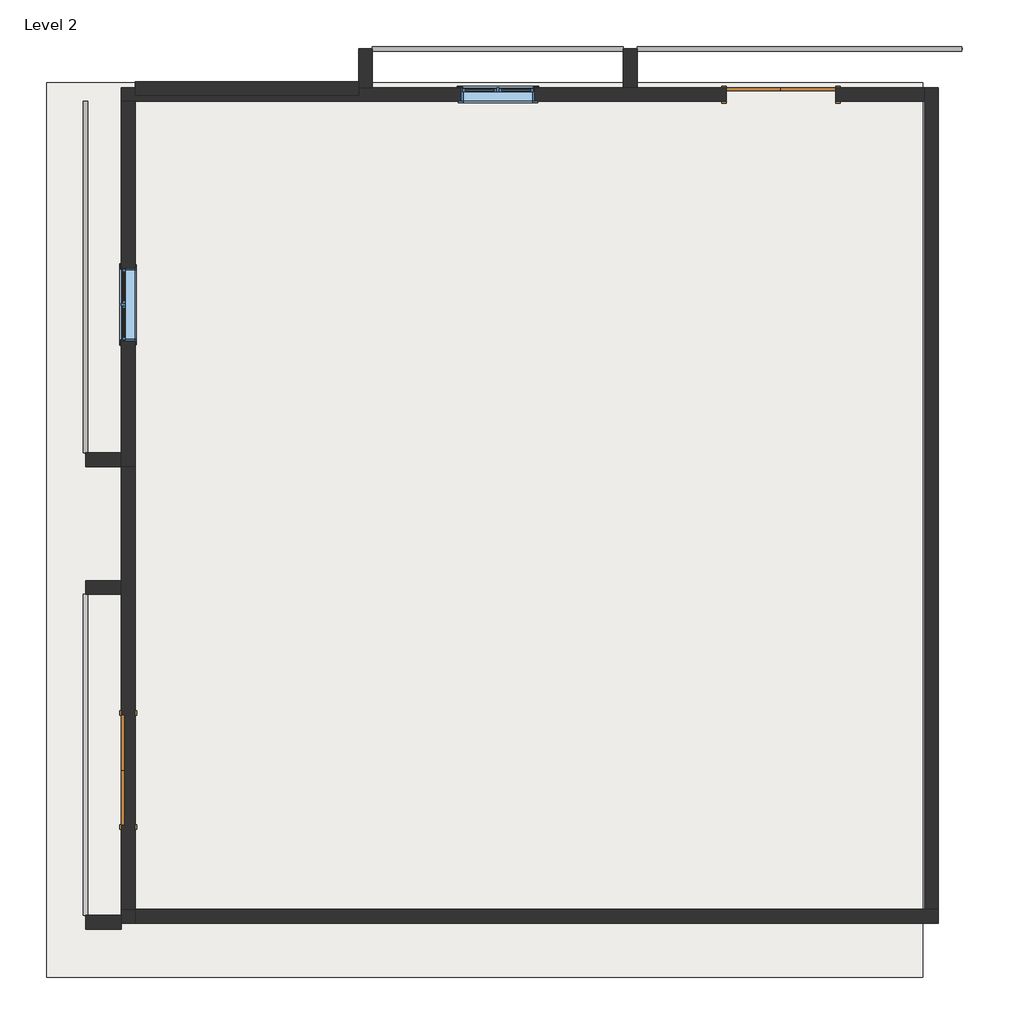
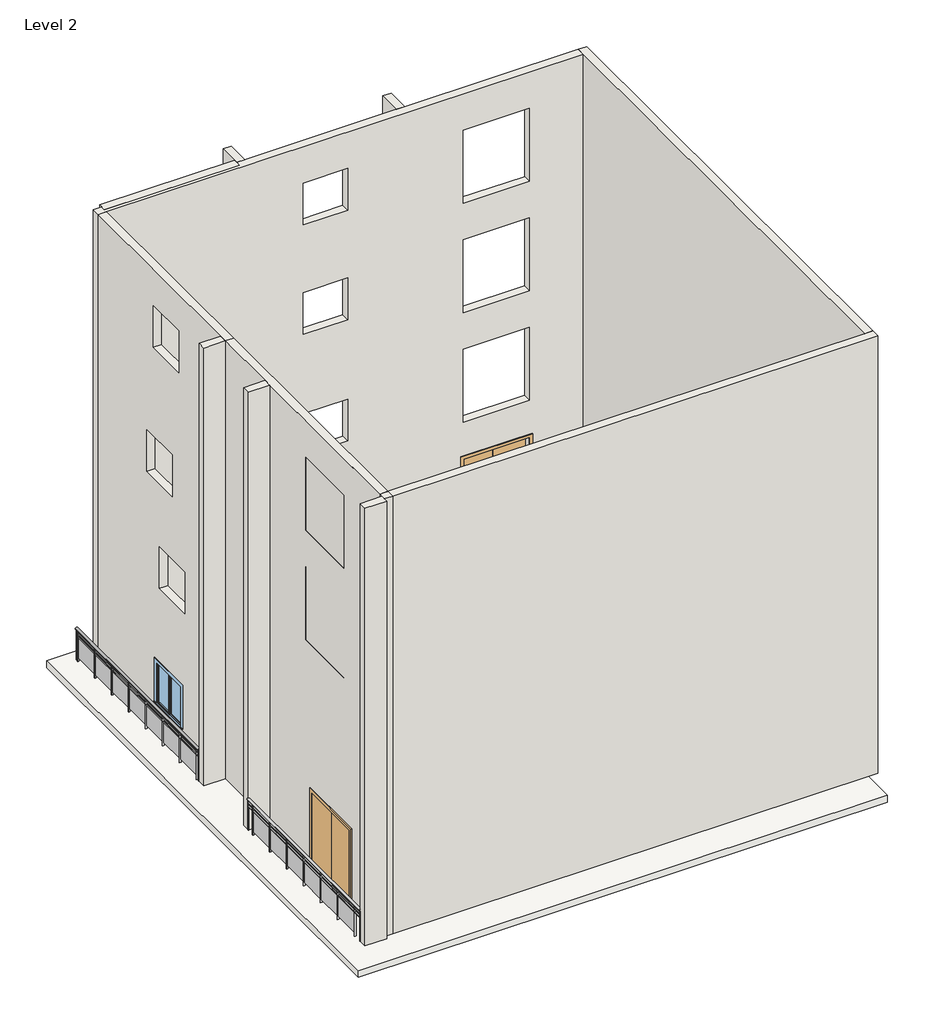
# One storey: 11 walls, 4 railings, 2 doors, 2 windows, 1 slab.
"""IFC4 building model written with IfcOpenShell, lengths in millimetres."""

from ifc_helpers import new_model, si_unit, point, frame, origin, place, context, project, spatial, polyline, ellipse_curve, trimmed, outline, extrude, faceted_brep, transform, mapped, element, save
from ifc_brep_helpers import plane_surface, extruded_surface, advanced_brep
from components import door_640b4634, window_534dcd48

model = new_model("IFC4")

# Units and contexts
model_context = context("Model", 3, world=origin())
ifc_project = project(units=[si_unit("LENGTHUNIT", "METRE", prefix="MILLI")], contexts=[model_context])

# Site, building, storey
site = spatial("IfcSite", under=ifc_project)
building = spatial("IfcBuilding", under=site)
storey = spatial("IfcBuildingStorey", under=building, Name="Level 2", Elevation=3200.4)

# Doors
placement = place(None, origin())
door_shape = door_640b4634(model_context)
element("IfcDoor", 1, ObjectType="Door-Double-Flush_Panel : 72\" x 84\"", at=placement, inside=storey, context=model_context, shape_type="MappedRepresentation", body=[
    mapped(door_shape, transform((-18468.543393, -7089.1397804, 3200.4), x_axis=(0.0, 1.0, 0.0), y_axis=(-1.0, 0.0, 0.0), z_axis=(0.0, 0.0, 1.0))),
])
element("IfcDoor", 2, ObjectType="Door-Double-Flush_Panel : 72\" x 84\"", at=placement, inside=storey, context=model_context, shape_type="MappedRepresentation", body=[
    mapped(door_shape, transform((-7571.943393, 4188.4602196, 3200.4), x_axis=(1.0, 0.0, 0.0), y_axis=(0.0, 1.0, 0.0), z_axis=(0.0, 0.0, 1.0))),
])

# Railings
element("IfcRailing", 3, ObjectType="Glass Panel - Bottom Fill", at=placement, inside=storey, context=model_context, shape_type="SolidModel", body=[
    advanced_brep(
    [(-19220.0296876, -9514.8397804, 4114.8), (-19143.8296876, -9514.8397804, 4114.8), (-19220.0296876, -4155.4397804, 4114.8), (-19143.8296876, -4155.4397804, 4114.8)],
    [
        (0, 1, ellipse_curve(frame((-19181.9296876, -9514.8397804, 4114.8), z_axis=(0.0, -1.0, 0.0), x_axis=(1.0, 0.0, 0.0)), 38.1, 28.575)),
        (1, 0, ellipse_curve(frame((-19181.9296876, -9514.8397804, 4114.8), z_axis=(0.0, -1.0, 0.0), x_axis=(1.0, 0.0, 0.0)), 38.1, 28.575)),
        (2, 3, ellipse_curve(frame((-19181.9296876, -4155.4397804, 4114.8), z_axis=(0.0, 1.0, 0.0), x_axis=(1.0, 0.0, 0.0)), 38.1, 28.575)),
        (3, 2, ellipse_curve(frame((-19181.9296876, -4155.4397804, 4114.8), z_axis=(0.0, 1.0, 0.0), x_axis=(1.0, 0.0, 0.0)), 38.1, 28.575)),
        (0, 2),
        (3, 1),
    ],
    [
        plane_surface(frame((-19181.9296876, -9514.8397804, 4114.8), z_axis=(0.0, -1.0, 0.0), x_axis=(0.0, 0.0, 1.0))),
        plane_surface(frame((-19181.9296876, -4155.4397804, 4114.8), z_axis=(0.0, 1.0, 0.0), x_axis=(0.0, 0.0, 1.0))),
        extruded_surface(trimmed(ellipse_curve(frame((-19181.9296876, -4155.4397804, 4114.8), z_axis=(0.0, -1.0, 0.0), x_axis=(1.0, 0.0, 0.0)), 38.1, 28.575), [point((-19220.0296876, -4155.4397804, 4114.8))], [point((-19143.8296876, -4155.4397804, 4114.8))], True, "CARTESIAN"), (0.0, -5359.4, 0.0), 5359.4),
        extruded_surface(trimmed(ellipse_curve(frame((-19181.9296876, -4155.4397804, 4114.8), z_axis=(0.0, -1.0, 0.0), x_axis=(1.0, 0.0, 0.0)), 38.1, 28.575), [point((-19143.8296876, -4155.4397804, 4114.8))], [point((-19220.0296876, -4155.4397804, 4114.8))], True, "CARTESIAN"), (0.0, -5359.4, 0.0), 5359.4),
    ],
    [
        (0, [[1, 2]]),
        (1, [[3, 4]]),
        (2, [[-1, 5, -4, 6]]),
        (3, [[-2, -6, -3, -5]]),
    ],
),
    extrude(outline(polyline([(-19169.2296876, -9514.8397804), (-19194.6296876, -9514.8397804), (-19194.6296876, -4155.4397804), (-19169.2296876, -4155.4397804), (-19169.2296876, -9514.8397804)])), frame((0.0, 0.0, 4000.5), z_axis=(0.0, 0.0, 1.0), x_axis=(1.0, 0.0, 0.0)), (0.0, 0.0, 1.0), 25.4),
    extrude(outline(polyline([(-19169.2296876, -9514.8397804), (-19194.6296876, -9514.8397804), (-19194.6296876, -4155.4397804), (-19169.2296876, -4155.4397804), (-19169.2296876, -9514.8397804)])), frame((0.0, 0.0, 3898.9), z_axis=(0.0, 0.0, 1.0), x_axis=(1.0, 0.0, 0.0)), (0.0, 0.0, 1.0), 25.4),
    extrude(outline(polyline([(-19156.5296876, -4403.0897804), (-19207.3296876, -4403.0897804), (-19207.3296876, -4390.3897804), (-19156.5296876, -4390.3897804), (-19156.5296876, -4403.0897804)])), frame((0.0, 0.0, 3200.4), z_axis=(0.0, 0.0, 1.0), x_axis=(1.0, 0.0, 0.0)), (0.0, 0.0, 1.0), 885.6788223),
    extrude(outline(polyline([(-19188.4648446, -5209.5397804), (-19188.4648446, -4396.7397804), (-19182.1148446, -4396.7397804), (-19182.1148446, -5209.5397804), (-19188.4648446, -5209.5397804)])), frame((0.0, 0.0, 3302.0), z_axis=(0.0, 0.0, 1.0), x_axis=(1.0, 0.0, 0.0)), (0.0, 0.0, 1.0), 596.9),
    extrude(outline(polyline([(-19156.5296876, -5215.8897804), (-19207.3296876, -5215.8897804), (-19207.3296876, -5203.1897804), (-19156.5296876, -5203.1897804), (-19156.5296876, -5215.8897804)])), frame((0.0, 0.0, 3200.4), z_axis=(0.0, 0.0, 1.0), x_axis=(1.0, 0.0, 0.0)), (0.0, 0.0, 1.0), 885.6788223),
    extrude(outline(polyline([(-19188.4648446, -6022.3397804), (-19188.4648446, -5209.5397804), (-19182.1148446, -5209.5397804), (-19182.1148446, -6022.3397804), (-19188.4648446, -6022.3397804)])), frame((0.0, 0.0, 3302.0), z_axis=(0.0, 0.0, 1.0), x_axis=(1.0, 0.0, 0.0)), (0.0, 0.0, 1.0), 596.9),
    extrude(outline(polyline([(-19156.5296876, -6028.6897804), (-19207.3296876, -6028.6897804), (-19207.3296876, -6015.9897804), (-19156.5296876, -6015.9897804), (-19156.5296876, -6028.6897804)])), frame((0.0, 0.0, 3200.4), z_axis=(0.0, 0.0, 1.0), x_axis=(1.0, 0.0, 0.0)), (0.0, 0.0, 1.0), 885.6788223),
    extrude(outline(polyline([(-19188.4648446, -6835.1397804), (-19188.4648446, -6022.3397804), (-19182.1148446, -6022.3397804), (-19182.1148446, -6835.1397804), (-19188.4648446, -6835.1397804)])), frame((0.0, 0.0, 3302.0), z_axis=(0.0, 0.0, 1.0), x_axis=(1.0, 0.0, 0.0)), (0.0, 0.0, 1.0), 596.9),
    extrude(outline(polyline([(-19156.5296876, -6841.4897804), (-19207.3296876, -6841.4897804), (-19207.3296876, -6828.7897804), (-19156.5296876, -6828.7897804), (-19156.5296876, -6841.4897804)])), frame((0.0, 0.0, 3200.4), z_axis=(0.0, 0.0, 1.0), x_axis=(1.0, 0.0, 0.0)), (0.0, 0.0, 1.0), 885.6788223),
    extrude(outline(polyline([(-19188.4648446, -7647.9397804), (-19188.4648446, -6835.1397804), (-19182.1148446, -6835.1397804), (-19182.1148446, -7647.9397804), (-19188.4648446, -7647.9397804)])), frame((0.0, 0.0, 3302.0), z_axis=(0.0, 0.0, 1.0), x_axis=(1.0, 0.0, 0.0)), (0.0, 0.0, 1.0), 596.9),
    extrude(outline(polyline([(-19156.5296876, -7654.2897804), (-19207.3296876, -7654.2897804), (-19207.3296876, -7641.5897804), (-19156.5296876, -7641.5897804), (-19156.5296876, -7654.2897804)])), frame((0.0, 0.0, 3200.4), z_axis=(0.0, 0.0, 1.0), x_axis=(1.0, 0.0, 0.0)), (0.0, 0.0, 1.0), 885.6788223),
    extrude(outline(polyline([(-19188.4648446, -8460.7397804), (-19188.4648446, -7647.9397804), (-19182.1148446, -7647.9397804), (-19182.1148446, -8460.7397804), (-19188.4648446, -8460.7397804)])), frame((0.0, 0.0, 3302.0), z_axis=(0.0, 0.0, 1.0), x_axis=(1.0, 0.0, 0.0)), (0.0, 0.0, 1.0), 596.9),
    extrude(outline(polyline([(-19156.5296876, -8467.0897804), (-19207.3296876, -8467.0897804), (-19207.3296876, -8454.3897804), (-19156.5296876, -8454.3897804), (-19156.5296876, -8467.0897804)])), frame((0.0, 0.0, 3200.4), z_axis=(0.0, 0.0, 1.0), x_axis=(1.0, 0.0, 0.0)), (0.0, 0.0, 1.0), 885.6788223),
    extrude(outline(polyline([(-19188.4648446, -9273.5397804), (-19188.4648446, -8460.7397804), (-19182.1148446, -8460.7397804), (-19182.1148446, -9273.5397804), (-19188.4648446, -9273.5397804)])), frame((0.0, 0.0, 3302.0), z_axis=(0.0, 0.0, 1.0), x_axis=(1.0, 0.0, 0.0)), (0.0, 0.0, 1.0), 596.9),
    extrude(outline(polyline([(-19156.5296876, -9279.8897804), (-19207.3296876, -9279.8897804), (-19207.3296876, -9267.1897804), (-19156.5296876, -9267.1897804), (-19156.5296876, -9279.8897804)])), frame((0.0, 0.0, 3200.4), z_axis=(0.0, 0.0, 1.0), x_axis=(1.0, 0.0, 0.0)), (0.0, 0.0, 1.0), 885.6788223),
    extrude(outline(polyline([(-19172.4046876, -4168.1397804), (-19191.4546876, -4168.1397804), (-19191.4546876, -4149.0897804), (-19172.4046876, -4149.0897804), (-19172.4046876, -4168.1397804)])), frame((0.0, 0.0, 3200.4), z_axis=(0.0, 0.0, 1.0), x_axis=(1.0, 0.0, 0.0)), (0.0, 0.0, 1.0), 885.6788223),
    extrude(outline(polyline([(-19172.4046876, -9521.1897804), (-19191.4546876, -9521.1897804), (-19191.4546876, -9502.1397804), (-19172.4046876, -9502.1397804), (-19172.4046876, -9521.1897804)])), frame((0.0, 0.0, 3200.4), z_axis=(0.0, 0.0, 1.0), x_axis=(1.0, 0.0, 0.0)), (0.0, 0.0, 1.0), 885.6788223),
])
element("IfcRailing", 4, ObjectType="Glass Panel - Bottom Fill", at=placement, inside=storey, context=model_context, shape_type="SolidModel", body=[
    advanced_brep(
    [(-19143.8296876, 4074.1602196, 4114.8), (-19220.0296876, 4074.1602196, 4114.8), (-19143.8296876, -1793.2397804, 4114.8), (-19220.0296876, -1793.2397804, 4114.8)],
    [
        (0, 1, ellipse_curve(frame((-19181.9296876, 4074.1602196, 4114.8), z_axis=(0.0, 1.0, 0.0), x_axis=(-1.0, 0.0, 0.0)), 38.1, 28.575)),
        (1, 0, ellipse_curve(frame((-19181.9296876, 4074.1602196, 4114.8), z_axis=(0.0, 1.0, 0.0), x_axis=(-1.0, 0.0, 0.0)), 38.1, 28.575)),
        (2, 3, ellipse_curve(frame((-19181.9296876, -1793.2397804, 4114.8), z_axis=(0.0, -1.0, 0.0), x_axis=(-1.0, 0.0, 0.0)), 38.1, 28.575)),
        (3, 2, ellipse_curve(frame((-19181.9296876, -1793.2397804, 4114.8), z_axis=(0.0, -1.0, 0.0), x_axis=(-1.0, 0.0, 0.0)), 38.1, 28.575)),
        (0, 2),
        (3, 1),
    ],
    [
        plane_surface(frame((-19181.9296876, 4074.1602196, 4114.8), z_axis=(0.0, 1.0, 0.0), x_axis=(0.0, 0.0, -1.0))),
        plane_surface(frame((-19181.9296876, -1793.2397804, 4114.8), z_axis=(0.0, -1.0, 0.0), x_axis=(0.0, 0.0, -1.0))),
        extruded_surface(trimmed(ellipse_curve(frame((-19181.9296876, -1793.2397804, 4114.8), z_axis=(0.0, 1.0, 0.0), x_axis=(-1.0, 0.0, 0.0)), 38.1, 28.575), [point((-19143.8296876, -1793.2397804, 4114.8))], [point((-19220.0296876, -1793.2397804, 4114.8))], True, "CARTESIAN"), (0.0, 5867.4, 0.0), 5867.4),
        extruded_surface(trimmed(ellipse_curve(frame((-19181.9296876, -1793.2397804, 4114.8), z_axis=(0.0, 1.0, 0.0), x_axis=(-1.0, 0.0, 0.0)), 38.1, 28.575), [point((-19220.0296876, -1793.2397804, 4114.8))], [point((-19143.8296876, -1793.2397804, 4114.8))], True, "CARTESIAN"), (0.0, 5867.4, 0.0), 5867.4),
    ],
    [
        (0, [[1, 2]]),
        (1, [[3, 4]]),
        (2, [[-1, 5, -4, 6]]),
        (3, [[-2, -6, -3, -5]]),
    ],
),
    extrude(outline(polyline([(-19194.6296876, 4074.1602196), (-19169.2296876, 4074.1602196), (-19169.2296876, -1793.2397804), (-19194.6296876, -1793.2397804), (-19194.6296876, 4074.1602196)])), frame((0.0, 0.0, 4000.5), z_axis=(0.0, 0.0, 1.0), x_axis=(1.0, 0.0, 0.0)), (0.0, 0.0, 1.0), 25.4),
    extrude(outline(polyline([(-19194.6296876, 4074.1602196), (-19169.2296876, 4074.1602196), (-19169.2296876, -1793.2397804), (-19194.6296876, -1793.2397804), (-19194.6296876, 4074.1602196)])), frame((0.0, 0.0, 3898.9), z_axis=(0.0, 0.0, 1.0), x_axis=(1.0, 0.0, 0.0)), (0.0, 0.0, 1.0), 25.4),
    extrude(outline(polyline([(-19207.3296876, -1697.9897804), (-19156.5296876, -1697.9897804), (-19156.5296876, -1710.6897804), (-19207.3296876, -1710.6897804), (-19207.3296876, -1697.9897804)])), frame((0.0, 0.0, 3200.4), z_axis=(0.0, 0.0, 1.0), x_axis=(1.0, 0.0, 0.0)), (0.0, 0.0, 1.0), 885.6788223),
    extrude(outline(polyline([(-19175.3945306, -891.5397804), (-19175.3945306, -1704.3397804), (-19181.7445306, -1704.3397804), (-19181.7445306, -891.5397804), (-19175.3945306, -891.5397804)])), frame((0.0, 0.0, 3302.0), z_axis=(0.0, 0.0, 1.0), x_axis=(1.0, 0.0, 0.0)), (0.0, 0.0, 1.0), 596.9),
    extrude(outline(polyline([(-19207.3296876, -885.1897804), (-19156.5296876, -885.1897804), (-19156.5296876, -897.8897804), (-19207.3296876, -897.8897804), (-19207.3296876, -885.1897804)])), frame((0.0, 0.0, 3200.4), z_axis=(0.0, 0.0, 1.0), x_axis=(1.0, 0.0, 0.0)), (0.0, 0.0, 1.0), 885.6788223),
    extrude(outline(polyline([(-19175.3945306, -78.7397804), (-19175.3945306, -891.5397804), (-19181.7445306, -891.5397804), (-19181.7445306, -78.7397804), (-19175.3945306, -78.7397804)])), frame((0.0, 0.0, 3302.0), z_axis=(0.0, 0.0, 1.0), x_axis=(1.0, 0.0, 0.0)), (0.0, 0.0, 1.0), 596.9),
    extrude(outline(polyline([(-19207.3296876, -72.3897804), (-19156.5296876, -72.3897804), (-19156.5296876, -85.0897804), (-19207.3296876, -85.0897804), (-19207.3296876, -72.3897804)])), frame((0.0, 0.0, 3200.4), z_axis=(0.0, 0.0, 1.0), x_axis=(1.0, 0.0, 0.0)), (0.0, 0.0, 1.0), 885.6788223),
    extrude(outline(polyline([(-19175.3945306, 734.0602196), (-19175.3945306, -78.7397804), (-19181.7445306, -78.7397804), (-19181.7445306, 734.0602196), (-19175.3945306, 734.0602196)])), frame((0.0, 0.0, 3302.0), z_axis=(0.0, 0.0, 1.0), x_axis=(1.0, 0.0, 0.0)), (0.0, 0.0, 1.0), 596.9),
    extrude(outline(polyline([(-19207.3296876, 740.4102196), (-19156.5296876, 740.4102196), (-19156.5296876, 727.7102196), (-19207.3296876, 727.7102196), (-19207.3296876, 740.4102196)])), frame((0.0, 0.0, 3200.4), z_axis=(0.0, 0.0, 1.0), x_axis=(1.0, 0.0, 0.0)), (0.0, 0.0, 1.0), 885.6788223),
    extrude(outline(polyline([(-19175.3945306, 1546.8602196), (-19175.3945306, 734.0602196), (-19181.7445306, 734.0602196), (-19181.7445306, 1546.8602196), (-19175.3945306, 1546.8602196)])), frame((0.0, 0.0, 3302.0), z_axis=(0.0, 0.0, 1.0), x_axis=(1.0, 0.0, 0.0)), (0.0, 0.0, 1.0), 596.9),
    extrude(outline(polyline([(-19207.3296876, 1553.2102196), (-19156.5296876, 1553.2102196), (-19156.5296876, 1540.5102196), (-19207.3296876, 1540.5102196), (-19207.3296876, 1553.2102196)])), frame((0.0, 0.0, 3200.4), z_axis=(0.0, 0.0, 1.0), x_axis=(1.0, 0.0, 0.0)), (0.0, 0.0, 1.0), 885.6788223),
    extrude(outline(polyline([(-19175.3945306, 2359.6602196), (-19175.3945306, 1546.8602196), (-19181.7445306, 1546.8602196), (-19181.7445306, 2359.6602196), (-19175.3945306, 2359.6602196)])), frame((0.0, 0.0, 3302.0), z_axis=(0.0, 0.0, 1.0), x_axis=(1.0, 0.0, 0.0)), (0.0, 0.0, 1.0), 596.9),
    extrude(outline(polyline([(-19207.3296876, 2366.0102196), (-19156.5296876, 2366.0102196), (-19156.5296876, 2353.3102196), (-19207.3296876, 2353.3102196), (-19207.3296876, 2366.0102196)])), frame((0.0, 0.0, 3200.4), z_axis=(0.0, 0.0, 1.0), x_axis=(1.0, 0.0, 0.0)), (0.0, 0.0, 1.0), 885.6788223),
    extrude(outline(polyline([(-19175.3945306, 3172.4602196), (-19175.3945306, 2359.6602196), (-19181.7445306, 2359.6602196), (-19181.7445306, 3172.4602196), (-19175.3945306, 3172.4602196)])), frame((0.0, 0.0, 3302.0), z_axis=(0.0, 0.0, 1.0), x_axis=(1.0, 0.0, 0.0)), (0.0, 0.0, 1.0), 596.9),
    extrude(outline(polyline([(-19207.3296876, 3178.8102196), (-19156.5296876, 3178.8102196), (-19156.5296876, 3166.1102196), (-19207.3296876, 3166.1102196), (-19207.3296876, 3178.8102196)])), frame((0.0, 0.0, 3200.4), z_axis=(0.0, 0.0, 1.0), x_axis=(1.0, 0.0, 0.0)), (0.0, 0.0, 1.0), 885.6788223),
    extrude(outline(polyline([(-19175.3945306, 3985.2602196), (-19175.3945306, 3172.4602196), (-19181.7445306, 3172.4602196), (-19181.7445306, 3985.2602196), (-19175.3945306, 3985.2602196)])), frame((0.0, 0.0, 3302.0), z_axis=(0.0, 0.0, 1.0), x_axis=(1.0, 0.0, 0.0)), (0.0, 0.0, 1.0), 596.9),
    extrude(outline(polyline([(-19207.3296876, 3991.6102196), (-19156.5296876, 3991.6102196), (-19156.5296876, 3978.9102196), (-19207.3296876, 3978.9102196), (-19207.3296876, 3991.6102196)])), frame((0.0, 0.0, 3200.4), z_axis=(0.0, 0.0, 1.0), x_axis=(1.0, 0.0, 0.0)), (0.0, 0.0, 1.0), 885.6788223),
    extrude(outline(polyline([(-19191.4546876, -1780.5397804), (-19172.4046876, -1780.5397804), (-19172.4046876, -1799.5897804), (-19191.4546876, -1799.5897804), (-19191.4546876, -1780.5397804)])), frame((0.0, 0.0, 3200.4), z_axis=(0.0, 0.0, 1.0), x_axis=(1.0, 0.0, 0.0)), (0.0, 0.0, 1.0), 885.6788223),
    extrude(outline(polyline([(-19191.4546876, 4080.5102196), (-19172.4046876, 4080.5102196), (-19172.4046876, 4061.4602196), (-19191.4546876, 4061.4602196), (-19191.4546876, 4080.5102196)])), frame((0.0, 0.0, 3200.4), z_axis=(0.0, 0.0, 1.0), x_axis=(1.0, 0.0, 0.0)), (0.0, 0.0, 1.0), 885.6788223),
])
element("IfcRailing", 5, ObjectType="Glass Panel - Bottom Fill", at=placement, inside=storey, context=model_context, shape_type="SolidModel", body=[
    advanced_brep(
    [(-14391.843393, 4991.4940048, 4114.8), (-14391.843393, 4915.2940048, 4114.8), (-10200.843393, 4991.4940048, 4114.8), (-10200.843393, 4915.2940048, 4114.8)],
    [
        (0, 1, ellipse_curve(frame((-14391.843393, 4953.3940048, 4114.8), z_axis=(-1.0, 0.0, 0.0), x_axis=(0.0, -1.0, 0.0)), 38.1, 28.575)),
        (1, 0, ellipse_curve(frame((-14391.843393, 4953.3940048, 4114.8), z_axis=(-1.0, 0.0, 0.0), x_axis=(0.0, -1.0, 0.0)), 38.1, 28.575)),
        (2, 3, ellipse_curve(frame((-10200.843393, 4953.3940048, 4114.8), z_axis=(1.0, 0.0, 0.0), x_axis=(0.0, -1.0, 0.0)), 38.1, 28.575)),
        (3, 2, ellipse_curve(frame((-10200.843393, 4953.3940048, 4114.8), z_axis=(1.0, 0.0, 0.0), x_axis=(0.0, -1.0, 0.0)), 38.1, 28.575)),
        (0, 2),
        (3, 1),
    ],
    [
        plane_surface(frame((-14391.843393, 4953.3940048, 4114.8), z_axis=(-1.0, 0.0, 0.0), x_axis=(0.0, 1.0, 0.0))),
        plane_surface(frame((-10200.843393, 4953.3940048, 4114.8), z_axis=(1.0, 0.0, 0.0), x_axis=(0.0, 1.0, 0.0))),
        extruded_surface(trimmed(ellipse_curve(frame((-10200.843393, 4953.3940048, 4114.8), z_axis=(-1.0, 0.0, 0.0), x_axis=(0.0, -1.0, 0.0)), 38.1, 28.575), [point((-10200.843393, 4991.4940048, 4114.8))], [point((-10200.843393, 4915.2940048, 4114.8))], True, "CARTESIAN"), (-4191.0, 0.0, 0.0), 4191.0),
        extruded_surface(trimmed(ellipse_curve(frame((-10200.843393, 4953.3940048, 4114.8), z_axis=(-1.0, 0.0, 0.0), x_axis=(0.0, -1.0, 0.0)), 38.1, 28.575), [point((-10200.843393, 4915.2940048, 4114.8))], [point((-10200.843393, 4991.4940048, 4114.8))], True, "CARTESIAN"), (-4191.0, 0.0, 0.0), 4191.0),
    ],
    [
        (0, [[1, 2]]),
        (1, [[3, 4]]),
        (2, [[-1, 5, -4, 6]]),
        (3, [[-2, -6, -3, -5]]),
    ],
),
    extrude(outline(polyline([(-14391.843393, 4940.6940048), (-14391.843393, 4966.0940048), (-10200.843393, 4966.0940048), (-10200.843393, 4940.6940048), (-14391.843393, 4940.6940048)])), frame((0.0, 0.0, 4000.5), z_axis=(0.0, 0.0, 1.0), x_axis=(1.0, 0.0, 0.0)), (0.0, 0.0, 1.0), 25.4),
    extrude(outline(polyline([(-14391.843393, 4940.6940048), (-14391.843393, 4966.0940048), (-10200.843393, 4966.0940048), (-10200.843393, 4940.6940048), (-14391.843393, 4940.6940048)])), frame((0.0, 0.0, 3898.9), z_axis=(0.0, 0.0, 1.0), x_axis=(1.0, 0.0, 0.0)), (0.0, 0.0, 1.0), 25.4),
    extrude(outline(polyline([(-10270.693393, 4927.9940048), (-10270.693393, 4978.7940048), (-10257.993393, 4978.7940048), (-10257.993393, 4927.9940048), (-10270.693393, 4927.9940048)])), frame((0.0, 0.0, 3200.4), z_axis=(0.0, 0.0, 1.0), x_axis=(1.0, 0.0, 0.0)), (0.0, 0.0, 1.0), 885.6788223),
    extrude(outline(polyline([(-11077.143393, 4959.9291618), (-10264.343393, 4959.9291618), (-10264.343393, 4953.5791618), (-11077.143393, 4953.5791618), (-11077.143393, 4959.9291618)])), frame((0.0, 0.0, 3302.0), z_axis=(0.0, 0.0, 1.0), x_axis=(1.0, 0.0, 0.0)), (0.0, 0.0, 1.0), 596.9),
    extrude(outline(polyline([(-11083.493393, 4927.9940048), (-11083.493393, 4978.7940048), (-11070.793393, 4978.7940048), (-11070.793393, 4927.9940048), (-11083.493393, 4927.9940048)])), frame((0.0, 0.0, 3200.4), z_axis=(0.0, 0.0, 1.0), x_axis=(1.0, 0.0, 0.0)), (0.0, 0.0, 1.0), 885.6788223),
    extrude(outline(polyline([(-11889.943393, 4959.9291618), (-11077.143393, 4959.9291618), (-11077.143393, 4953.5791618), (-11889.943393, 4953.5791618), (-11889.943393, 4959.9291618)])), frame((0.0, 0.0, 3302.0), z_axis=(0.0, 0.0, 1.0), x_axis=(1.0, 0.0, 0.0)), (0.0, 0.0, 1.0), 596.9),
    extrude(outline(polyline([(-11896.293393, 4927.9940048), (-11896.293393, 4978.7940048), (-11883.593393, 4978.7940048), (-11883.593393, 4927.9940048), (-11896.293393, 4927.9940048)])), frame((0.0, 0.0, 3200.4), z_axis=(0.0, 0.0, 1.0), x_axis=(1.0, 0.0, 0.0)), (0.0, 0.0, 1.0), 885.6788223),
    extrude(outline(polyline([(-12702.743393, 4959.9291618), (-11889.943393, 4959.9291618), (-11889.943393, 4953.5791618), (-12702.743393, 4953.5791618), (-12702.743393, 4959.9291618)])), frame((0.0, 0.0, 3302.0), z_axis=(0.0, 0.0, 1.0), x_axis=(1.0, 0.0, 0.0)), (0.0, 0.0, 1.0), 596.9),
    extrude(outline(polyline([(-12709.093393, 4927.9940048), (-12709.093393, 4978.7940048), (-12696.393393, 4978.7940048), (-12696.393393, 4927.9940048), (-12709.093393, 4927.9940048)])), frame((0.0, 0.0, 3200.4), z_axis=(0.0, 0.0, 1.0), x_axis=(1.0, 0.0, 0.0)), (0.0, 0.0, 1.0), 885.6788223),
    extrude(outline(polyline([(-13515.543393, 4959.9291618), (-12702.743393, 4959.9291618), (-12702.743393, 4953.5791618), (-13515.543393, 4953.5791618), (-13515.543393, 4959.9291618)])), frame((0.0, 0.0, 3302.0), z_axis=(0.0, 0.0, 1.0), x_axis=(1.0, 0.0, 0.0)), (0.0, 0.0, 1.0), 596.9),
    extrude(outline(polyline([(-13521.893393, 4927.9940048), (-13521.893393, 4978.7940048), (-13509.193393, 4978.7940048), (-13509.193393, 4927.9940048), (-13521.893393, 4927.9940048)])), frame((0.0, 0.0, 3200.4), z_axis=(0.0, 0.0, 1.0), x_axis=(1.0, 0.0, 0.0)), (0.0, 0.0, 1.0), 885.6788223),
    extrude(outline(polyline([(-14328.343393, 4959.9291618), (-13515.543393, 4959.9291618), (-13515.543393, 4953.5791618), (-14328.343393, 4953.5791618), (-14328.343393, 4959.9291618)])), frame((0.0, 0.0, 3302.0), z_axis=(0.0, 0.0, 1.0), x_axis=(1.0, 0.0, 0.0)), (0.0, 0.0, 1.0), 596.9),
    extrude(outline(polyline([(-14334.693393, 4927.9940048), (-14334.693393, 4978.7940048), (-14321.993393, 4978.7940048), (-14321.993393, 4927.9940048), (-14334.693393, 4927.9940048)])), frame((0.0, 0.0, 3200.4), z_axis=(0.0, 0.0, 1.0), x_axis=(1.0, 0.0, 0.0)), (0.0, 0.0, 1.0), 885.6788223),
    extrude(outline(polyline([(-10213.543393, 4943.8690048), (-10213.543393, 4962.9190048), (-10194.493393, 4962.9190048), (-10194.493393, 4943.8690048), (-10213.543393, 4943.8690048)])), frame((0.0, 0.0, 3200.4), z_axis=(0.0, 0.0, 1.0), x_axis=(1.0, 0.0, 0.0)), (0.0, 0.0, 1.0), 885.6788223),
    extrude(outline(polyline([(-14398.193393, 4943.8690048), (-14398.193393, 4962.9190048), (-14379.143393, 4962.9190048), (-14379.143393, 4943.8690048), (-14398.193393, 4943.8690048)])), frame((0.0, 0.0, 3200.4), z_axis=(0.0, 0.0, 1.0), x_axis=(1.0, 0.0, 0.0)), (0.0, 0.0, 1.0), 885.6788223),
])
element("IfcRailing", 6, ObjectType="Glass Panel - Bottom Fill", at=placement, inside=storey, context=model_context, shape_type="SolidModel", body=[
    advanced_brep(
    [(-9972.243393, 4991.4940048, 4114.8), (-9972.243393, 4915.2940048, 4114.8), (-4551.5296876, 4991.4940048, 4114.8), (-4551.5296876, 4915.2940048, 4114.8)],
    [
        (0, 1, ellipse_curve(frame((-9972.243393, 4953.3940048, 4114.8), z_axis=(-1.0, 0.0, 0.0), x_axis=(0.0, -1.0, 0.0)), 38.1, 28.575)),
        (1, 0, ellipse_curve(frame((-9972.243393, 4953.3940048, 4114.8), z_axis=(-1.0, 0.0, 0.0), x_axis=(0.0, -1.0, 0.0)), 38.1, 28.575)),
        (2, 3, ellipse_curve(frame((-4551.5296876, 4953.3940048, 4114.8), z_axis=(1.0, 0.0, 0.0), x_axis=(0.0, -1.0, 0.0)), 38.1, 28.575)),
        (3, 2, ellipse_curve(frame((-4551.5296876, 4953.3940048, 4114.8), z_axis=(1.0, 0.0, 0.0), x_axis=(0.0, -1.0, 0.0)), 38.1, 28.575)),
        (0, 2),
        (3, 1),
    ],
    [
        plane_surface(frame((-9972.243393, 4953.3940048, 4114.8), z_axis=(-1.0, 0.0, 0.0), x_axis=(0.0, 1.0, 0.0))),
        plane_surface(frame((-4551.5296876, 4953.3940048, 4114.8), z_axis=(1.0, 0.0, 0.0), x_axis=(0.0, 1.0, 0.0))),
        extruded_surface(trimmed(ellipse_curve(frame((-4551.5296876, 4953.3940048, 4114.8), z_axis=(-1.0, 0.0, 0.0), x_axis=(0.0, -1.0, 0.0)), 38.1, 28.575), [point((-4551.5296876, 4991.4940048, 4114.8))], [point((-4551.5296876, 4915.2940048, 4114.8))], True, "CARTESIAN"), (-5420.7137054, 0.0, 0.0), 5420.7137054),
        extruded_surface(trimmed(ellipse_curve(frame((-4551.5296876, 4953.3940048, 4114.8), z_axis=(-1.0, 0.0, 0.0), x_axis=(0.0, -1.0, 0.0)), 38.1, 28.575), [point((-4551.5296876, 4915.2940048, 4114.8))], [point((-4551.5296876, 4991.4940048, 4114.8))], True, "CARTESIAN"), (-5420.7137054, 0.0, 0.0), 5420.7137054),
    ],
    [
        (0, [[1, 2]]),
        (1, [[3, 4]]),
        (2, [[-1, 5, -4, 6]]),
        (3, [[-2, -6, -3, -5]]),
    ],
),
    extrude(outline(polyline([(-9972.243393, 4940.6940048), (-9972.243393, 4966.0940048), (-4551.5296876, 4966.0940048), (-4551.5296876, 4940.6940048), (-9972.243393, 4940.6940048)])), frame((0.0, 0.0, 4000.5), z_axis=(0.0, 0.0, 1.0), x_axis=(1.0, 0.0, 0.0)), (0.0, 0.0, 1.0), 25.4),
    extrude(outline(polyline([(-9972.243393, 4940.6940048), (-9972.243393, 4966.0940048), (-4551.5296876, 4966.0940048), (-4551.5296876, 4940.6940048), (-9972.243393, 4940.6940048)])), frame((0.0, 0.0, 3898.9), z_axis=(0.0, 0.0, 1.0), x_axis=(1.0, 0.0, 0.0)), (0.0, 0.0, 1.0), 25.4),
    extrude(outline(polyline([(-4829.8365403, 4927.9940048), (-4829.8365403, 4978.7940048), (-4817.1365403, 4978.7940048), (-4817.1365403, 4927.9940048), (-4829.8365403, 4927.9940048)])), frame((0.0, 0.0, 3200.4), z_axis=(0.0, 0.0, 1.0), x_axis=(1.0, 0.0, 0.0)), (0.0, 0.0, 1.0), 885.6788223),
    extrude(outline(polyline([(-5636.2865403, 4959.9291618), (-4823.4865403, 4959.9291618), (-4823.4865403, 4953.5791618), (-5636.2865403, 4953.5791618), (-5636.2865403, 4959.9291618)])), frame((0.0, 0.0, 3302.0), z_axis=(0.0, 0.0, 1.0), x_axis=(1.0, 0.0, 0.0)), (0.0, 0.0, 1.0), 596.9),
    extrude(outline(polyline([(-5642.6365403, 4927.9940048), (-5642.6365403, 4978.7940048), (-5629.9365403, 4978.7940048), (-5629.9365403, 4927.9940048), (-5642.6365403, 4927.9940048)])), frame((0.0, 0.0, 3200.4), z_axis=(0.0, 0.0, 1.0), x_axis=(1.0, 0.0, 0.0)), (0.0, 0.0, 1.0), 885.6788223),
    extrude(outline(polyline([(-6449.0865403, 4959.9291618), (-5636.2865403, 4959.9291618), (-5636.2865403, 4953.5791618), (-6449.0865403, 4953.5791618), (-6449.0865403, 4959.9291618)])), frame((0.0, 0.0, 3302.0), z_axis=(0.0, 0.0, 1.0), x_axis=(1.0, 0.0, 0.0)), (0.0, 0.0, 1.0), 596.9),
    extrude(outline(polyline([(-6455.4365403, 4927.9940048), (-6455.4365403, 4978.7940048), (-6442.7365403, 4978.7940048), (-6442.7365403, 4927.9940048), (-6455.4365403, 4927.9940048)])), frame((0.0, 0.0, 3200.4), z_axis=(0.0, 0.0, 1.0), x_axis=(1.0, 0.0, 0.0)), (0.0, 0.0, 1.0), 885.6788223),
    extrude(outline(polyline([(-7261.8865403, 4959.9291618), (-6449.0865403, 4959.9291618), (-6449.0865403, 4953.5791618), (-7261.8865403, 4953.5791618), (-7261.8865403, 4959.9291618)])), frame((0.0, 0.0, 3302.0), z_axis=(0.0, 0.0, 1.0), x_axis=(1.0, 0.0, 0.0)), (0.0, 0.0, 1.0), 596.9),
    extrude(outline(polyline([(-7268.2365403, 4927.9940048), (-7268.2365403, 4978.7940048), (-7255.5365403, 4978.7940048), (-7255.5365403, 4927.9940048), (-7268.2365403, 4927.9940048)])), frame((0.0, 0.0, 3200.4), z_axis=(0.0, 0.0, 1.0), x_axis=(1.0, 0.0, 0.0)), (0.0, 0.0, 1.0), 885.6788223),
    extrude(outline(polyline([(-8074.6865403, 4959.9291618), (-7261.8865403, 4959.9291618), (-7261.8865403, 4953.5791618), (-8074.6865403, 4953.5791618), (-8074.6865403, 4959.9291618)])), frame((0.0, 0.0, 3302.0), z_axis=(0.0, 0.0, 1.0), x_axis=(1.0, 0.0, 0.0)), (0.0, 0.0, 1.0), 596.9),
    extrude(outline(polyline([(-8081.0365403, 4927.9940048), (-8081.0365403, 4978.7940048), (-8068.3365403, 4978.7940048), (-8068.3365403, 4927.9940048), (-8081.0365403, 4927.9940048)])), frame((0.0, 0.0, 3200.4), z_axis=(0.0, 0.0, 1.0), x_axis=(1.0, 0.0, 0.0)), (0.0, 0.0, 1.0), 885.6788223),
    extrude(outline(polyline([(-8887.4865403, 4959.9291618), (-8074.6865403, 4959.9291618), (-8074.6865403, 4953.5791618), (-8887.4865403, 4953.5791618), (-8887.4865403, 4959.9291618)])), frame((0.0, 0.0, 3302.0), z_axis=(0.0, 0.0, 1.0), x_axis=(1.0, 0.0, 0.0)), (0.0, 0.0, 1.0), 596.9),
    extrude(outline(polyline([(-8893.8365403, 4927.9940048), (-8893.8365403, 4978.7940048), (-8881.1365403, 4978.7940048), (-8881.1365403, 4927.9940048), (-8893.8365403, 4927.9940048)])), frame((0.0, 0.0, 3200.4), z_axis=(0.0, 0.0, 1.0), x_axis=(1.0, 0.0, 0.0)), (0.0, 0.0, 1.0), 885.6788223),
    extrude(outline(polyline([(-9700.2865403, 4959.9291618), (-8887.4865403, 4959.9291618), (-8887.4865403, 4953.5791618), (-9700.2865403, 4953.5791618), (-9700.2865403, 4959.9291618)])), frame((0.0, 0.0, 3302.0), z_axis=(0.0, 0.0, 1.0), x_axis=(1.0, 0.0, 0.0)), (0.0, 0.0, 1.0), 596.9),
    extrude(outline(polyline([(-9706.6365403, 4927.9940048), (-9706.6365403, 4978.7940048), (-9693.9365403, 4978.7940048), (-9693.9365403, 4927.9940048), (-9706.6365403, 4927.9940048)])), frame((0.0, 0.0, 3200.4), z_axis=(0.0, 0.0, 1.0), x_axis=(1.0, 0.0, 0.0)), (0.0, 0.0, 1.0), 885.6788223),
    extrude(outline(polyline([(-4564.2296876, 4943.8690048), (-4564.2296876, 4962.9190048), (-4545.1796876, 4962.9190048), (-4545.1796876, 4943.8690048), (-4564.2296876, 4943.8690048)])), frame((0.0, 0.0, 3200.4), z_axis=(0.0, 0.0, 1.0), x_axis=(1.0, 0.0, 0.0)), (0.0, 0.0, 1.0), 885.6788223),
    extrude(outline(polyline([(-9978.593393, 4943.8690048), (-9978.593393, 4962.9190048), (-9959.543393, 4962.9190048), (-9959.543393, 4943.8690048), (-9978.593393, 4943.8690048)])), frame((0.0, 0.0, 3200.4), z_axis=(0.0, 0.0, 1.0), x_axis=(1.0, 0.0, 0.0)), (0.0, 0.0, 1.0), 885.6788223),
])

# Slab
element("IfcSlab", 7, ObjectType="Generic - 12\"", at=placement, inside=storey, context=model_context, shape_type="SweptSolid", body=[
    extrude(outline(polyline([(-5202.5726551, 4385.0703181), (-5202.5726551, -10550.1296819), (-19832.9726551, -10550.1296819), (-19832.9726551, 4385.0703181), (-5202.5726551, 4385.0703181)])), frame((0.0, 0.0, 2997.2), z_axis=(0.0, 0.0, 1.0), x_axis=(1.0, 0.0, 0.0)), (0.0, 0.0, 1.0), 203.2),
])

# Walls
element("IfcWall", 8, ObjectType="Generic - 8\"", at=placement, inside=storey, context=model_context, shape_type="Brep", body=[
    faceted_brep([(-5171.643393, 4074.1602196, 16002.0), (-18354.243393, 4074.1602196, 16002.0), (-18582.843393, 4074.1602196, 16002.0), (-18582.843393, 4074.1602196, 3200.4), (-18354.243393, 4074.1602196, 3200.4), (-8486.343393, 4074.1602196, 3200.4), (-8486.343393, 4074.1602196, 5334.0), (-6657.543393, 4074.1602196, 5334.0), (-6657.543393, 4074.1602196, 3200.4), (-5171.643393, 4074.1602196, 3200.4), (-6657.543393, 4074.1602196, 12801.6), (-8486.343393, 4074.1602196, 12801.6), (-8486.343393, 4074.1602196, 14935.2), (-6657.543393, 4074.1602196, 14935.2), (-6657.543393, 4074.1602196, 9601.2), (-8486.343393, 4074.1602196, 9601.2), (-8486.343393, 4074.1602196, 11734.8), (-6657.543393, 4074.1602196, 11734.8), (-6657.543393, 4074.1602196, 6400.8), (-8486.343393, 4074.1602196, 6400.8), (-8486.343393, 4074.1602196, 8534.4), (-6657.543393, 4074.1602196, 8534.4), (-11686.743393, 4074.1602196, 14935.2), (-11686.743393, 4074.1602196, 13716.0), (-12905.943393, 4074.1602196, 13716.0), (-12905.943393, 4074.1602196, 14935.2), (-11686.743393, 4074.1602196, 11734.8), (-11686.743393, 4074.1602196, 10515.6), (-12905.943393, 4074.1602196, 10515.6), (-12905.943393, 4074.1602196, 11734.8), (-11686.743393, 4074.1602196, 8191.8927979), (-11686.743393, 4074.1602196, 6972.6927979), (-12905.943393, 4074.1602196, 6972.6927979), (-12905.943393, 4074.1602196, 8191.8927979), (-11686.743393, 4074.1602196, 5334.0), (-11686.743393, 4074.1602196, 4114.8), (-12905.943393, 4074.1602196, 4114.8), (-12905.943393, 4074.1602196, 5334.0), (-18582.843393, 4302.7602196, 16002.0), (-14620.443393, 4302.7602196, 16002.0), (-14391.843393, 4302.7602196, 16002.0), (-10200.843393, 4302.7602196, 16002.0), (-9972.243393, 4302.7602196, 16002.0), (-5171.643393, 4302.7602196, 16002.0), (-5171.643393, 4302.7602196, 3200.4), (-6657.543393, 4302.7602196, 3200.4), (-6657.543393, 4302.7602196, 5334.0), (-8486.343393, 4302.7602196, 5334.0), (-8486.343393, 4302.7602196, 3200.4), (-9972.243393, 4302.7602196, 3200.4), (-10200.843393, 4302.7602196, 3200.4), (-14391.843393, 4302.7602196, 3200.4), (-14620.443393, 4302.7602196, 3200.4), (-18582.843393, 4302.7602196, 3200.4), (-6657.543393, 4302.7602196, 12801.6), (-6657.543393, 4302.7602196, 14935.2), (-8486.343393, 4302.7602196, 14935.2), (-8486.343393, 4302.7602196, 12801.6), (-6657.543393, 4302.7602196, 9601.2), (-6657.543393, 4302.7602196, 11734.8), (-8486.343393, 4302.7602196, 11734.8), (-8486.343393, 4302.7602196, 9601.2), (-6657.543393, 4302.7602196, 6400.8), (-6657.543393, 4302.7602196, 8534.4), (-8486.343393, 4302.7602196, 8534.4), (-8486.343393, 4302.7602196, 6400.8), (-11686.743393, 4302.7602196, 14935.2), (-12905.943393, 4302.7602196, 14935.2), (-12905.943393, 4302.7602196, 13716.0), (-11686.743393, 4302.7602196, 13716.0), (-11686.743393, 4302.7602196, 11734.8), (-12905.943393, 4302.7602196, 11734.8), (-12905.943393, 4302.7602196, 10515.6), (-11686.743393, 4302.7602196, 10515.6), (-11686.743393, 4302.7602196, 8191.8927979), (-12905.943393, 4302.7602196, 8191.8927979), (-12905.943393, 4302.7602196, 6972.6927979), (-11686.743393, 4302.7602196, 6972.6927979), (-11686.743393, 4302.7602196, 5334.0), (-12905.943393, 4302.7602196, 5334.0), (-12905.943393, 4302.7602196, 4114.8), (-11686.743393, 4302.7602196, 4114.8)], [[[0, 1, 2, 3, 4, 5, 6, 7, 8, 9], [10, 11, 12, 13], [14, 15, 16, 17], [18, 19, 20, 21], [22, 23, 24, 25], [26, 27, 28, 29], [30, 31, 32, 33], [34, 35, 36, 37]], [[38, 39, 40, 41, 42, 43, 44, 45, 46, 47, 48, 49, 50, 51, 52, 53], [54, 55, 56, 57], [58, 59, 60, 61], [62, 63, 64, 65], [66, 67, 68, 69], [70, 71, 72, 73], [74, 75, 76, 77], [78, 79, 80, 81]], [[3, 53, 52, 51, 50, 49, 48, 5, 4]], [[44, 9, 8, 45]], [[2, 1, 0, 43, 42, 41, 40, 39, 38]], [[3, 2, 38, 53]], [[0, 9, 44, 43]], [[55, 54, 10, 13]], [[56, 55, 13, 12]], [[57, 56, 12, 11]], [[54, 57, 11, 10]], [[59, 58, 14, 17]], [[60, 59, 17, 16]], [[61, 60, 16, 15]], [[58, 61, 15, 14]], [[63, 62, 18, 21]], [[64, 63, 21, 20]], [[65, 64, 20, 19]], [[62, 65, 19, 18]], [[7, 46, 45, 8]], [[46, 7, 6, 47]], [[47, 6, 5, 48]], [[23, 22, 66, 69]], [[24, 23, 69, 68]], [[25, 24, 68, 67]], [[22, 25, 67, 66]], [[27, 26, 70, 73]], [[28, 27, 73, 72]], [[29, 28, 72, 71]], [[26, 29, 71, 70]], [[31, 30, 74, 77]], [[32, 31, 77, 76]], [[33, 32, 76, 75]], [[30, 33, 75, 74]], [[35, 34, 78, 81]], [[36, 35, 81, 80]], [[37, 36, 80, 79]], [[34, 37, 79, 78]]]),
])
element("IfcWall", 9, ObjectType="Generic - 8\"", at=placement, inside=storey, context=model_context, shape_type="Brep", body=[
    faceted_brep([(-18354.243393, 4074.1602196, 16002.0), (-18354.243393, -9413.2397804, 16002.0), (-18354.243393, -9641.8397804, 16002.0), (-18354.243393, -9641.8397804, 3200.4), (-18354.243393, -9413.2397804, 3200.4), (-18354.243393, -8003.5397804, 3200.4), (-18354.243393, -8003.5397804, 5334.0), (-18354.243393, -6174.7397804, 5334.0), (-18354.243393, -6174.7397804, 3200.4), (-18354.243393, 4074.1602196, 3200.4), (-18354.243393, 1292.8602196, 4634.2879893), (-18354.243393, 1292.8602196, 3415.0879893), (-18354.243393, 73.6602196, 3415.0879893), (-18354.243393, 73.6602196, 4634.2879893), (-18354.243393, 1140.4602196, 8066.6186704), (-18354.243393, 1140.4602196, 6847.4186704), (-18354.243393, -78.7397804, 6847.4186704), (-18354.243393, -78.7397804, 8066.6186704), (-18354.243393, 1750.0602196, 11119.8811016), (-18354.243393, 1750.0602196, 9900.6811016), (-18354.243393, 530.8602196, 9900.6811016), (-18354.243393, 530.8602196, 11119.8811016), (-18354.243393, 1445.2602196, 14935.2), (-18354.243393, 1445.2602196, 13716.0), (-18354.243393, 226.0602196, 13716.0), (-18354.243393, 226.0602196, 14935.2), (-18354.243393, -6174.7397804, 6400.8), (-18354.243393, -8003.5397804, 6400.8), (-18354.243393, -8003.5397804, 8534.4), (-18354.243393, -6174.7397804, 8534.4), (-18354.243393, -5869.9397804, 9601.2), (-18354.243393, -7698.7397804, 9601.2), (-18354.243393, -7698.7397804, 11734.8), (-18354.243393, -5869.9397804, 11734.8), (-18582.843393, -9641.8397804, 16002.0), (-18582.843393, -9514.8397804, 16002.0), (-18582.843393, -4155.4397804, 16002.0), (-18582.843393, -3926.8397804, 16002.0), (-18582.843393, -2021.8397804, 16002.0), (-18582.843393, -1793.2397804, 16002.0), (-18582.843393, 4074.1602196, 16002.0), (-18582.843393, 4074.1602196, 3200.4), (-18582.843393, -1793.2397804, 3200.4), (-18582.843393, -2021.8397804, 3200.4), (-18582.843393, -3926.8397804, 3200.4), (-18582.843393, -4155.4397804, 3200.4), (-18582.843393, -6174.7397804, 3200.4), (-18582.843393, -6174.7397804, 5334.0), (-18582.843393, -8003.5397804, 5334.0), (-18582.843393, -8003.5397804, 3200.4), (-18582.843393, -9514.8397804, 3200.4), (-18582.843393, -9641.8397804, 3200.4), (-18582.843393, 1292.8602196, 4634.2879893), (-18582.843393, 73.6602196, 4634.2879893), (-18582.843393, 73.6602196, 3415.0879893), (-18582.843393, 1292.8602196, 3415.0879893), (-18582.843393, 1140.4602196, 8066.6186704), (-18582.843393, -78.7397804, 8066.6186704), (-18582.843393, -78.7397804, 6847.4186704), (-18582.843393, 1140.4602196, 6847.4186704), (-18582.843393, 1750.0602196, 11119.8811016), (-18582.843393, 530.8602196, 11119.8811016), (-18582.843393, 530.8602196, 9900.6811016), (-18582.843393, 1750.0602196, 9900.6811016), (-18582.843393, 1445.2602196, 14935.2), (-18582.843393, 226.0602196, 14935.2), (-18582.843393, 226.0602196, 13716.0), (-18582.843393, 1445.2602196, 13716.0), (-18582.843393, -6174.7397804, 6400.8), (-18582.843393, -6174.7397804, 8534.4), (-18582.843393, -8003.5397804, 8534.4), (-18582.843393, -8003.5397804, 6400.8), (-18582.843393, -5869.9397804, 9601.2), (-18582.843393, -5869.9397804, 11734.8), (-18582.843393, -7698.7397804, 11734.8), (-18582.843393, -7698.7397804, 9601.2)], [[[0, 1, 2, 3, 4, 5, 6, 7, 8, 9], [10, 11, 12, 13], [14, 15, 16, 17], [18, 19, 20, 21], [22, 23, 24, 25], [26, 27, 28, 29], [30, 31, 32, 33]], [[34, 35, 36, 37, 38, 39, 40, 41, 42, 43, 44, 45, 46, 47, 48, 49, 50, 51], [52, 53, 54, 55], [56, 57, 58, 59], [60, 61, 62, 63], [64, 65, 66, 67], [68, 69, 70, 71], [72, 73, 74, 75]], [[3, 51, 50, 49, 5, 4]], [[41, 9, 8, 46, 45, 44, 43, 42]], [[2, 1, 0, 40, 39, 38, 37, 36, 35, 34]], [[3, 2, 34, 51]], [[0, 9, 41, 40]], [[11, 10, 52, 55]], [[12, 11, 55, 54]], [[13, 12, 54, 53]], [[10, 13, 53, 52]], [[15, 14, 56, 59]], [[16, 15, 59, 58]], [[17, 16, 58, 57]], [[14, 17, 57, 56]], [[19, 18, 60, 63]], [[20, 19, 63, 62]], [[21, 20, 62, 61]], [[18, 21, 61, 60]], [[23, 22, 64, 67]], [[24, 23, 67, 66]], [[25, 24, 66, 65]], [[22, 25, 65, 64]], [[69, 68, 26, 29]], [[70, 69, 29, 28]], [[71, 70, 28, 27]], [[68, 71, 27, 26]], [[7, 47, 46, 8]], [[47, 7, 6, 48]], [[48, 6, 5, 49]], [[73, 72, 30, 33]], [[74, 73, 33, 32]], [[75, 74, 32, 31]], [[72, 75, 31, 30]]]),
])
element("IfcWall", 10, ObjectType="Generic - 8\"", at=placement, inside=storey, context=model_context, shape_type="Brep", body=[
    faceted_brep([(-4943.043393, -9413.2397804, 3200.4), (-5171.643393, -9413.2397804, 3200.4), (-18354.243393, -9413.2397804, 3200.4), (-18354.243393, -9413.2397804, 16002.0), (-5171.643393, -9413.2397804, 16002.0), (-4943.043393, -9413.2397804, 16002.0), (-4943.043393, -9641.8397804, 3200.4), (-4943.043393, -9641.8397804, 16002.0), (-18354.243393, -9641.8397804, 16002.0), (-18354.243393, -9641.8397804, 3200.4)], [[[0, 1, 2, 3, 4, 5]], [[6, 7, 8, 9]], [[2, 1, 0, 6, 9]], [[5, 4, 3, 8, 7]], [[0, 5, 7, 6]], [[3, 2, 9, 8]]]),
])
element("IfcWall", 11, ObjectType="Generic - 8\"", at=placement, inside=storey, context=model_context, shape_type="Brep", body=[
    faceted_brep([(-5171.643393, 4302.7602196, 3200.4), (-5171.643393, 4074.1602196, 3200.4), (-5171.643393, -9413.2397804, 3200.4), (-5171.643393, -9413.2397804, 16002.0), (-5171.643393, 4074.1602196, 16002.0), (-5171.643393, 4302.7602196, 16002.0), (-4943.043393, 4302.7602196, 3200.4), (-4943.043393, 4302.7602196, 16002.0), (-4943.043393, -9413.2397804, 16002.0), (-4943.043393, -9413.2397804, 3200.4)], [[[0, 1, 2, 3, 4, 5]], [[6, 7, 8, 9]], [[2, 1, 0, 6, 9]], [[5, 4, 3, 8, 7]], [[0, 5, 7, 6]], [[3, 2, 9, 8]]]),
])
element("IfcWall", 12, ObjectType="Generic - 8\"", at=placement, inside=storey, context=model_context, shape_type="SweptSolid", body=[
    extrude(outline(polyline([(-18582.843393, -2021.8397804), (-19181.9296876, -2021.8397804), (-19181.9296876, -1793.2397804), (-18582.843393, -1793.2397804), (-18582.843393, -2021.8397804)])), frame((0.0, 0.0, 3200.4), z_axis=(0.0, 0.0, 1.0), x_axis=(1.0, 0.0, 0.0)), (0.0, 0.0, 1.0), 12801.6),
])
element("IfcWall", 13, ObjectType="Generic - 8\"", at=placement, inside=storey, context=model_context, shape_type="Brep", body=[
    faceted_brep([(-18354.243393, -9413.2397804, 3200.4), (-18354.243393, -2021.8397804, 3200.4), (-18354.243393, -2021.8397804, 16002.0), (-18354.243393, -9413.2397804, 16002.0), (-18354.243393, -5869.9397804, 12801.6), (-18354.243393, -7698.7397804, 12801.6), (-18354.243393, -7698.7397804, 14935.2), (-18354.243393, -5869.9397804, 14935.2), (-18582.843393, -9413.2397804, 3200.4), (-18582.843393, -9413.2397804, 16002.0), (-18582.843393, -4155.4397804, 16002.0), (-18582.843393, -3926.8397804, 16002.0), (-18582.843393, -2021.8397804, 16002.0), (-18582.843393, -2021.8397804, 3200.4), (-18582.843393, -3926.8397804, 3200.4), (-18582.843393, -4155.4397804, 3200.4), (-18582.843393, -5869.9397804, 12801.6), (-18582.843393, -5869.9397804, 14935.2), (-18582.843393, -7698.7397804, 14935.2), (-18582.843393, -7698.7397804, 12801.6)], [[[0, 1, 2, 3], [4, 5, 6, 7]], [[8, 9, 10, 11, 12, 13, 14, 15], [16, 17, 18, 19]], [[2, 1, 13, 12]], [[1, 0, 8, 15, 14, 13]], [[3, 2, 12, 11, 10, 9]], [[0, 3, 9, 8]], [[17, 16, 4, 7]], [[18, 17, 7, 6]], [[19, 18, 6, 5]], [[16, 19, 5, 4]]]),
])
element("IfcWall", 14, ObjectType="Generic - 8\"", at=placement, inside=storey, context=model_context, shape_type="Brep", body=[
    faceted_brep([(-18582.843393, -9514.8397804, 3200.4), (-19181.9296876, -9514.8397804, 3200.4), (-19181.9296876, -9514.8397804, 16002.0), (-18582.843393, -9514.8397804, 16002.0), (-18582.843393, -9743.4397804, 3200.4), (-18582.843393, -9743.4397804, 16002.0), (-19181.9296876, -9743.4397804, 16002.0), (-19181.9296876, -9743.4397804, 3200.4), (-18582.843393, -9641.8397804, 3200.4), (-18582.843393, -9641.8397804, 16002.0)], [[[0, 1, 2, 3]], [[4, 5, 6, 7]], [[1, 0, 8, 4, 7]], [[2, 1, 7, 6]], [[3, 2, 6, 5, 9]], [[0, 3, 9, 5, 4, 8]]]),
])
element("IfcWall", 15, ObjectType="Generic - 8\"", at=placement, inside=storey, context=model_context, shape_type="SweptSolid", body=[
    extrude(outline(polyline([(-18582.843393, -4155.4397804), (-19181.9296876, -4155.4397804), (-19181.9296876, -3926.8397804), (-18582.843393, -3926.8397804), (-18582.843393, -4155.4397804)])), frame((0.0, 0.0, 3200.4), z_axis=(0.0, 0.0, 1.0), x_axis=(1.0, 0.0, 0.0)), (0.0, 0.0, 1.0), 12801.6),
])
element("IfcWall", 16, ObjectType="Generic - 8\"", at=placement, inside=storey, context=model_context, shape_type="SweptSolid", body=[
    extrude(outline(polyline([(-9972.243393, 4953.3940048), (-9972.243393, 4302.7602196), (-10200.843393, 4302.7602196), (-10200.843393, 4953.3940048), (-9972.243393, 4953.3940048)])), frame((0.0, 0.0, 3200.4), z_axis=(0.0, 0.0, 1.0), x_axis=(1.0, 0.0, 0.0)), (0.0, 0.0, 1.0), 12801.6),
])
element("IfcWall", 17, ObjectType="Generic - 8\"", at=placement, inside=storey, context=model_context, shape_type="Brep", body=[
    faceted_brep([(-14391.843393, 4302.7602196, 3200.4), (-14391.843393, 4953.3940048, 3200.4), (-14391.843393, 4953.3940048, 16002.0), (-14391.843393, 4302.7602196, 16002.0), (-14620.443393, 4302.7602196, 3200.4), (-14620.443393, 4302.7602196, 16002.0), (-14620.443393, 4404.3602196, 16002.0), (-14620.443393, 4953.3940048, 16002.0), (-14620.443393, 4953.3940048, 3200.4), (-14620.443393, 4404.3602196, 3200.4)], [[[0, 1, 2, 3]], [[4, 5, 6, 7, 8, 9]], [[1, 0, 4, 9, 8]], [[2, 1, 8, 7]], [[3, 2, 7, 6, 5]], [[0, 3, 5, 4]]]),
])
element("IfcWall", 18, ObjectType="Generic - 8\"", at=placement, inside=storey, context=model_context, shape_type="Brep", body=[
    faceted_brep([(-14620.443393, 4404.3602196, 3200.4), (-18354.243393, 4404.3602196, 3200.4), (-18354.243393, 4404.3602196, 16002.0), (-14620.443393, 4404.3602196, 16002.0), (-14620.443393, 4175.7602196, 3200.4), (-14620.443393, 4175.7602196, 16002.0), (-18354.243393, 4175.7602196, 16002.0), (-18354.243393, 4175.7602196, 3200.4), (-14620.443393, 4302.7602196, 3200.4), (-14620.443393, 4302.7602196, 16002.0)], [[[0, 1, 2, 3]], [[4, 5, 6, 7]], [[1, 0, 8, 4, 7]], [[3, 2, 6, 5, 9]], [[0, 3, 9, 5, 4, 8]], [[2, 1, 7, 6]]]),
])

# Windows
window_shape = window_534dcd48(model_context)
element("IfcWindow", 19, ObjectType="Casement Dbl with Trim : 48\" x 48\"", at=placement, inside=storey, context=model_context, shape_type="MappedRepresentation", body=[
    mapped(window_shape, transform((-18449.493393, 683.2602196, 2500.6879893), x_axis=(0.0, 1.0, 0.0), y_axis=(-1.0, 0.0, 0.0), z_axis=(0.0, 0.0, 1.0))),
])
element("IfcWindow", 20, ObjectType="Casement Dbl with Trim : 48\" x 48\"", at=placement, inside=storey, context=model_context, shape_type="MappedRepresentation", body=[
    mapped(window_shape, transform((-12296.343393, 4169.4102196, 3200.4), x_axis=(1.0, 0.0, 0.0), y_axis=(0.0, 1.0, 0.0), z_axis=(0.0, 0.0, 1.0))),
])

save(model, "model.ifc")

# Revit data of these elements
# Type "Door-Double-Flush_Panel : 72\" x 84\""
#   Type Mark = "11"
#   Construction Type Id = "DOOR"
#   Assembly Code = "C1020"
#   Analytic Construction = "Wooden"
#   Thickness = 0' - 2"
#   Thermal Resistance (R) = 2.5876 (h·ft²·°F)/BTU
#   Swing Angle [instance default] = 90.00°
#   Panel Width = 3' - 0"
#   Heat Transfer Coefficient (U) = 0.3865 BTU/(h·ft²·°F)
#   Height = 7' - 0"
#   Trim Projection Ext = 0' - 1"
#   Trim Projection Int = 0' - 1"
#   Trim Width = 0' - 3"
#   Width = 6' - 0"
#   Define Thermal Properties by = 1
#   Panel Material = Glass, Clear Glazing
#   Trim Material = Paint - Sienna
#   Visual Light Transmittance = 0
#   Solar Heat Gain Coefficient = 0
#   Function = (empty or 0)
#   Wall Closure = (empty or 0)
# Type "Glass Panel - Bottom Fill"
#   Assembly Code = "C2010400"
#   built-in parameter 1008612 = 0.0416667 (stored number, unit not read)
#   built-in parameter 1008611 = 0.0416667 (stored number, unit not read)
#   built-in parameter 1008609 = 0.333333 (stored number, unit not read)
#   built-in parameter 1008604 = 0.166667 (stored number, unit not read)
#   built-in parameter 1008603 = 0.166667 (stored number, unit not read)
#   Railing Height = 3' - 0"
#   built-in parameter 1008630 = 2
#   built-in parameter 1008610 = 2
#   built-in parameter 1008618 = Baluster - Square : 3/4"
# Type "Generic - 12\""
#   Assembly Code = "B1010"
#   Function = 0
#   Layers, outside or top first: 0' - 8" no material (function 1)
# Type "Generic - 8\""
#   Assembly Code = "B2010"
#   Layers, outside or top first: 0' - 9" no material (function 1)
# Type "Casement Dbl with Trim : 48\" x 48\""
#   Type Mark = "10"
#   Construction Type Id = "GSP4R"
#   Assembly Code = "B2020100"
#   Analytic Construction = "1/8 in Pilkington single glazing"
#   Visual Light Transmittance = 0.9
#   Solar Heat Gain Coefficient = 0.78
#   Heat Transfer Coefficient (U) = 0.6496 BTU/(h·ft²·°F)
#   Height = 4' - 0"
#   Default Sill Height = 3' - 0"
#   Trim Projection - Ext. = 0' - 0 1/2"
#   Trim Projection - Int. = 0' - 0 3/4"
#   Trim Width - Exterior = 0' - 3 1/2"
#   Trim Width - Interior = 0' - 3 1/2"
#   Width = 4' - 0"
#   Window Inset = 0' - 0 3/4"
#   Define Thermal Properties by = 1
#   Glass Pane Material = Glass
#   Sash Material = Glass, Clear Glazing
#   Trim Exterior Material = Earth
#   Trim Interior Material = Trim
#   Wall Closure = (empty or 0)
# Elements 1, 2 (IfcDoor, "Door-Double-Flush_Panel : 72\" x 84\"")
#   Swing Angle = 90.00°
#   Phase Created = New Construction
#   Materials on its faces: "Paint - Sienna", "Glass, Clear Glazing"
# Elements 3, 4, 5, 6 (IfcRailing, "Glass Panel - Bottom Fill")
#   Phase Created = New Construction
#   Materials on its faces: "Glass"
# Element 7 (IfcSlab, "Generic - 12\"")
#   Height Offset From Level = 0' - 0"
#   Phase Created = New Construction
#   Materials on its faces: "Default Floor"
# Elements 8, 9, 10, 11, 12, 13, 14, 15, 16, 17, 18 (IfcWall, "Generic - 8\"")
#   Top Offset = 0' - 0"
#   Base Offset = 0' - 0"
#   Unconnected Height = 42' - 0"
#   wall height = 42' - 0"
#   Phase Created = New Construction
#   Base Constraint = Level 2
#   Materials on its faces: "Default Wall"
# Element 19 (IfcWindow, "Casement Dbl with Trim : 48\" x 48\"")
#   Mark = "1"
#   Phase Created = New Construction
#   Materials on its faces: "Glass, Clear Glazing", "Earth", "Glass", "Trim"
# Element 20 (IfcWindow, "Casement Dbl with Trim : 48\" x 48\"")
#   Mark = "8"
#   Phase Created = New Construction
#   Materials on its faces: "Glass, Clear Glazing", "Earth", "Glass", "Trim"
# Materials
#   "Glass, Clear Glazing": class "Glass", colour RGB 0 128 192, transparency 0.75, Description = "Clear glazing", Cost = 0
#   "Paint - Sienna": colour RGB 118 70 51, transparency 0, Cost = 0
#   "Glass": class "Glass", colour RGB 0 128 192, transparency 0.75, Description = "Soda Lime Glass", Cost = 0
#   "Earth": class "Generic", colour RGB 97 75 62, transparency 0, Description = "Soil", Cost = 0
#   "Trim": class "Wood", colour RGB 224 178 126, transparency 0
#   "Default Floor": colour RGB 128 128 128, transparency 0
#   "Default Wall": colour RGB 128 128 128, transparency 0
